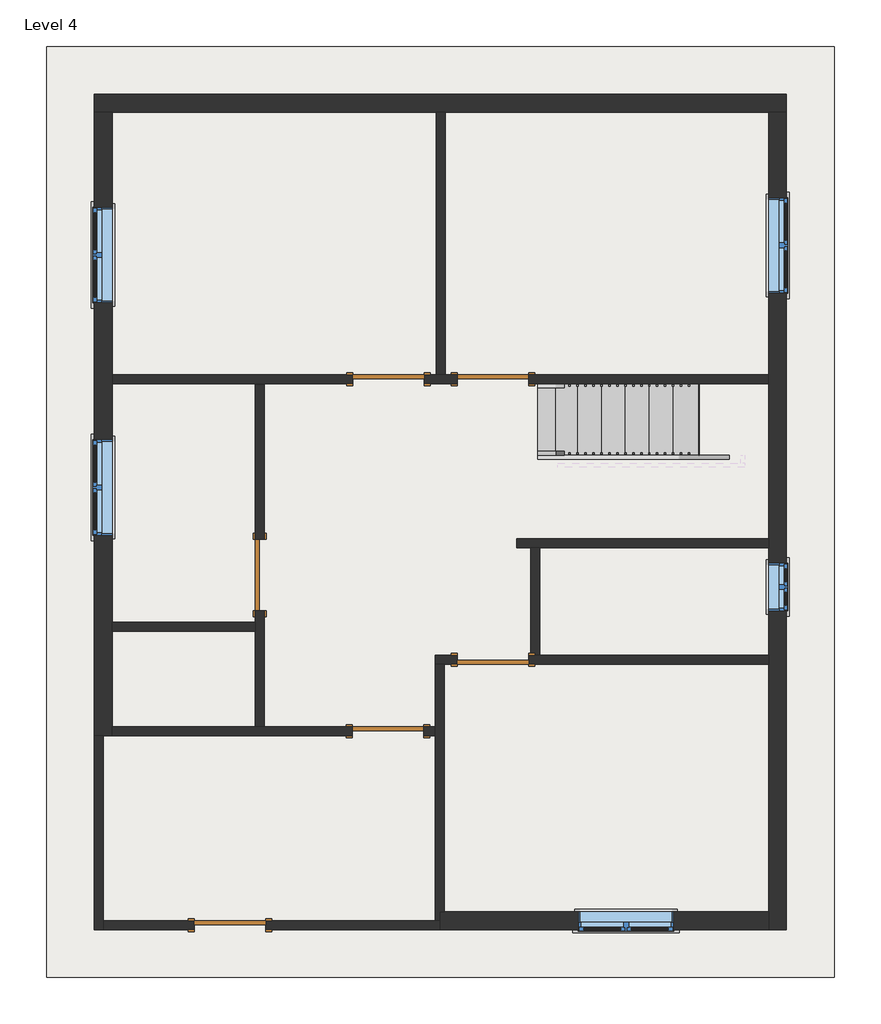
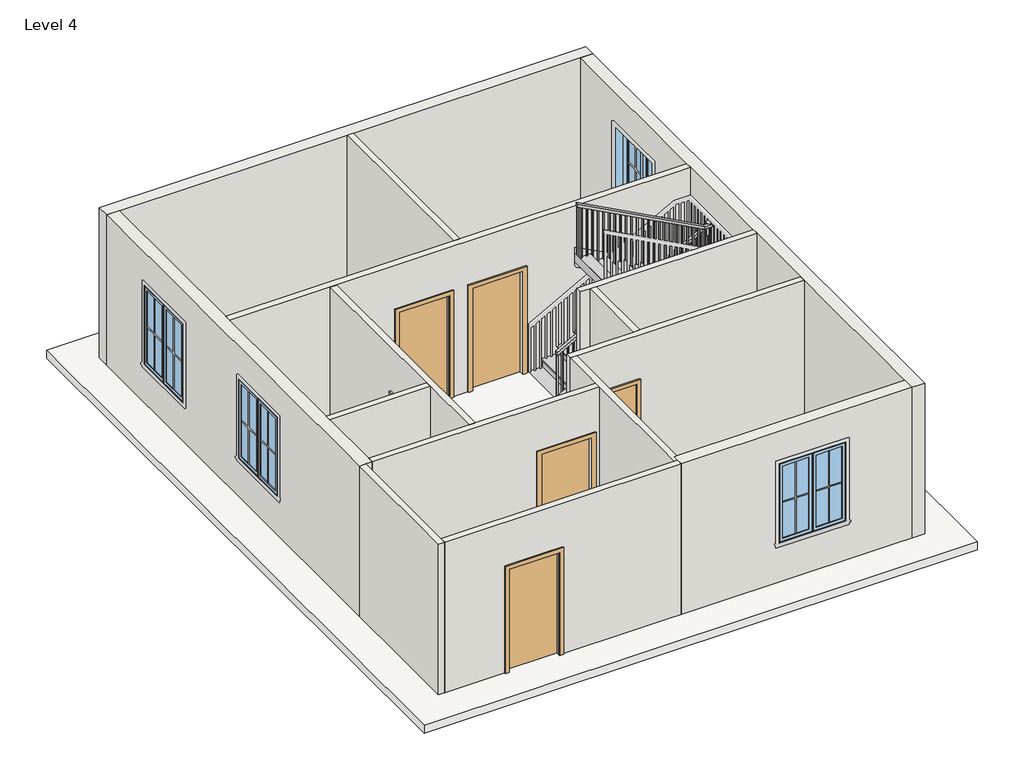
# One storey, part 1 of 2: 15 walls, 6 doors, 5 windows, 1 railing, 1 roof, 1 stair flight.
"""IFC4 building model written with IfcOpenShell, lengths in millimetres."""

from ifc_helpers import new_model, si_unit, frame, origin, place, context, project, spatial, polyline, outline, extrude, faceted_brep, transform, mapped, element, save
from components import door_305aa2a5, door_e5f9f3c4, stair_flight_cd99e03c, window_c417fced, window_8377141f

model = new_model("IFC4")

# Units and contexts
model_context = context("Model", 3, world=origin())
ifc_project = project(units=[si_unit("LENGTHUNIT", "METRE", prefix="MILLI")], contexts=[model_context])

# Site, building, storey
site = spatial("IfcSite", under=ifc_project)
building = spatial("IfcBuilding", under=site)
storey = spatial("IfcBuildingStorey", under=building, Name="Level 4", Elevation=9144.0)

# Doors
placement = place(None, origin())
door_shape = door_305aa2a5(model_context)
element("IfcDoor", 1, ObjectType="Single-Flush : 36\" x 84\"", at=placement, inside=storey, context=model_context, shape_type="MappedRepresentation", body=[
    mapped(door_shape, transform((8001.0, 9251.95, 9144.0), x_axis=(-1.0, 0.0, 0.0), y_axis=(0.0, -1.0, 0.0), z_axis=(0.0, 0.0, 1.0))),
])
element("IfcDoor", 2, ObjectType="Single-Flush : 36\" x 84\"", at=placement, inside=storey, context=model_context, shape_type="MappedRepresentation", body=[
    mapped(door_shape, transform((5022.9818578, 6750.05, 9144.0), x_axis=(0.0, -1.0, 0.0), y_axis=(1.0, 0.0, 0.0), z_axis=(0.0, 0.0, 1.0))),
])
door_2_shape = door_e5f9f3c4(model_context)
element("IfcDoor", 3, ObjectType="Single-Flush : 36\" x 84\"", at=placement, inside=storey, context=model_context, shape_type="MappedRepresentation", body=[
    mapped(door_2_shape, transform((6667.5, 9251.95, 9144.0), x_axis=(1.0, 0.0, 0.0), y_axis=(0.0, 1.0, 0.0), z_axis=(0.0, 0.0, 1.0))),
])
element("IfcDoor", 4, ObjectType="Single-Flush : 36\" x 84\"", at=placement, inside=storey, context=model_context, shape_type="MappedRepresentation", body=[
    mapped(door_2_shape, transform((8001.0, 5670.55, 9144.0), x_axis=(-1.0, 0.0, 0.0), y_axis=(0.0, -1.0, 0.0), z_axis=(0.0, 0.0, 1.0))),
])
element("IfcDoor", 5, ObjectType="Single-Flush : 36\" x 84\"", at=placement, inside=storey, context=model_context, shape_type="MappedRepresentation", body=[
    mapped(door_2_shape, transform((6658.76875, 4756.15, 9144.0), x_axis=(1.0, 0.0, 0.0), y_axis=(0.0, 1.0, 0.0), z_axis=(0.0, 0.0, 1.0))),
])
element("IfcDoor", 6, ObjectType="Single-Flush : 36\" x 84\"", at=placement, inside=storey, context=model_context, shape_type="MappedRepresentation", body=[
    mapped(door_2_shape, transform((4641.85, 2279.65, 9144.0), x_axis=(1.0, 0.0, 0.0), y_axis=(0.0, 1.0, 0.0), z_axis=(0.0, 0.0, 1.0))),
])

# Railing
element("IfcRailing", 7, ObjectType="Handrail - Rectangular", at=placement, inside=storey, context=model_context, shape_type="SolidModel", body=[
    faceted_brep([(8572.5, 8331.2, 10218.8210526), (8572.5, 8331.2, 10160.9285199), (8572.5, 8280.4, 10160.9285199), (8572.5, 8280.4, 10218.8210526), (11137.9, 8331.2, 11620.962753), (11188.7, 8331.2, 11590.8354025), (11188.7, 8280.4, 11590.8354025), (11137.9, 8280.4, 11620.962753), (11137.9, 8331.2, 11662.6105263), (11188.7, 8331.2, 11611.8105263), (11188.7, 8280.4, 11611.8105263), (11137.9, 8280.4, 11662.6105263), (11264.9, 8331.2, 11662.6105263), (11264.9, 8331.2, 11611.8105263), (11214.1, 8280.4, 11611.8105263), (11214.1, 8280.4, 11662.6105263), (11264.9, 8204.2, 11662.6105263), (11264.9, 8153.4, 11611.8105263), (11214.1, 8153.4, 11611.8105263), (11214.1, 8204.2, 11662.6105263), (11264.9, 8204.2, 11863.9901456), (11264.9, 8153.4, 11813.1901456), (11214.1, 8153.4, 11813.1901456), (11214.1, 8204.2, 11863.9901456), (11264.9, 8077.2, 11863.9901456), (11264.9, 8077.2, 11813.1901456), (11214.1, 8128.0, 11813.1901456), (11214.1, 8128.0, 11863.9901456), (11137.9, 8077.2, 11863.9901456), (11125.1122768, 8077.2, 11813.1901456), (11125.1122768, 8128.0, 11813.1901456), (11137.9, 8128.0, 11863.9901456), (8826.5, 8077.2, 13106.4), (8826.5, 8128.0, 13106.4), (8826.5, 8128.0, 13048.7264198), (8826.5, 8077.2, 13048.7264198)], [[[0, 1, 2, 3]], [[1, 0, 4, 5]], [[2, 1, 5, 6]], [[3, 2, 6, 7]], [[0, 3, 7, 4]], [[5, 4, 8, 9]], [[6, 5, 9, 10]], [[7, 6, 10, 11]], [[4, 7, 11, 8]], [[9, 8, 12, 13]], [[10, 9, 13, 14]], [[11, 10, 14, 15]], [[8, 11, 15, 12]], [[13, 12, 16, 17]], [[14, 13, 17, 18]], [[15, 14, 18, 19]], [[12, 15, 19, 16]], [[17, 16, 20, 21]], [[18, 17, 21, 22]], [[19, 18, 22, 23]], [[16, 19, 23, 20]], [[21, 20, 24, 25]], [[22, 21, 25, 26]], [[23, 22, 26, 27]], [[20, 23, 27, 24]], [[25, 24, 28, 29]], [[26, 25, 29, 30]], [[27, 26, 30, 31]], [[24, 27, 31, 28]], [[32, 33, 34, 35]], [[29, 28, 32, 35]], [[30, 29, 35, 34]], [[31, 30, 34, 33]], [[28, 31, 33, 32]]]),
    extrude(outline(polyline([(13002.6480323, 8912.225), (13012.887674, 8893.175), (12031.5789474, 8893.175), (12031.5789474, 8912.225), (13002.6480323, 8912.225)])), frame((0.0, 8093.075, 0.0), z_axis=(0.0, 1.0, 0.0), x_axis=(0.0, 0.0, 1.0)), (0.0, 0.0, 1.0), 19.05),
    extrude(outline(polyline([(12948.0366101, 9013.825), (12958.2762518, 8994.775), (12031.5789474, 8994.775), (12031.5789474, 9013.825), (12948.0366101, 9013.825)])), frame((0.0, 8093.075, 0.0), z_axis=(0.0, 1.0, 0.0), x_axis=(0.0, 0.0, 1.0)), (0.0, 0.0, 1.0), 19.05),
    extrude(outline(polyline([(12893.425188, 9115.425), (12903.6648296, 9096.375), (11871.1578947, 9096.375), (11871.1578947, 9115.425), (12893.425188, 9115.425)])), frame((0.0, 8093.075, 0.0), z_axis=(0.0, 1.0, 0.0), x_axis=(0.0, 0.0, 1.0)), (0.0, 0.0, 1.0), 19.05),
    extrude(outline(polyline([(12838.8137658, 9217.025), (12849.0534074, 9197.975), (11871.1578947, 9197.975), (11871.1578947, 9217.025), (12838.8137658, 9217.025)])), frame((0.0, 8093.075, 0.0), z_axis=(0.0, 1.0, 0.0), x_axis=(0.0, 0.0, 1.0)), (0.0, 0.0, 1.0), 19.05),
    extrude(outline(polyline([(12784.1597952, 9318.625), (12794.5717386, 9299.575), (11871.1578947, 9299.575), (11871.1578947, 9318.625), (12784.1597952, 9318.625)])), frame((0.0, 8093.075, 0.0), z_axis=(0.0, 1.0, 0.0), x_axis=(0.0, 0.0, 1.0)), (0.0, 0.0, 1.0), 19.05),
    extrude(outline(polyline([(12729.5909214, 9420.225), (12739.8305631, 9401.175), (11710.7368421, 9401.175), (11710.7368421, 9420.225), (12729.5909214, 9420.225)])), frame((0.0, 8093.075, 0.0), z_axis=(0.0, 1.0, 0.0), x_axis=(0.0, 0.0, 1.0)), (0.0, 0.0, 1.0), 19.05),
    extrude(outline(polyline([(12674.9794993, 9521.825), (12685.2191409, 9502.775), (11710.7368421, 9502.775), (11710.7368421, 9521.825), (12674.9794993, 9521.825)])), frame((0.0, 8093.075, 0.0), z_axis=(0.0, 1.0, 0.0), x_axis=(0.0, 0.0, 1.0)), (0.0, 0.0, 1.0), 19.05),
    extrude(outline(polyline([(12620.3680771, 9623.425), (12630.6077187, 9604.375), (11710.7368421, 9604.375), (11710.7368421, 9623.425), (12620.3680771, 9623.425)])), frame((0.0, 8093.075, 0.0), z_axis=(0.0, 1.0, 0.0), x_axis=(0.0, 0.0, 1.0)), (0.0, 0.0, 1.0), 19.05),
    extrude(outline(polyline([(12565.7566549, 9725.025), (12575.9962966, 9705.975), (11550.3157895, 9705.975), (11550.3157895, 9725.025), (12565.7566549, 9725.025)])), frame((0.0, 8093.075, 0.0), z_axis=(0.0, 1.0, 0.0), x_axis=(0.0, 0.0, 1.0)), (0.0, 0.0, 1.0), 19.05),
    extrude(outline(polyline([(12511.1452327, 9826.625), (12521.3848744, 9807.575), (11550.3157895, 9807.575), (11550.3157895, 9826.625), (12511.1452327, 9826.625)])), frame((0.0, 8093.075, 0.0), z_axis=(0.0, 1.0, 0.0), x_axis=(0.0, 0.0, 1.0)), (0.0, 0.0, 1.0), 19.05),
    extrude(outline(polyline([(12456.5338106, 9928.225), (12466.7734522, 9909.175), (11550.3157895, 9909.175), (11550.3157895, 9928.225), (12456.5338106, 9928.225)])), frame((0.0, 8093.075, 0.0), z_axis=(0.0, 1.0, 0.0), x_axis=(0.0, 0.0, 1.0)), (0.0, 0.0, 1.0), 19.05),
    extrude(outline(polyline([(12401.9223884, 10029.825), (12412.1620301, 10010.775), (11389.8947368, 10010.775), (11389.8947368, 10029.825), (12401.9223884, 10029.825)])), frame((0.0, 8093.075, 0.0), z_axis=(0.0, 1.0, 0.0), x_axis=(0.0, 0.0, 1.0)), (0.0, 0.0, 1.0), 19.05),
    extrude(outline(polyline([(12347.3109662, 10131.425), (12357.5506079, 10112.375), (11389.8947368, 10112.375), (11389.8947368, 10131.425), (12347.3109662, 10131.425)])), frame((0.0, 8093.075, 0.0), z_axis=(0.0, 1.0, 0.0), x_axis=(0.0, 0.0, 1.0)), (0.0, 0.0, 1.0), 19.05),
    extrude(outline(polyline([(12292.6995441, 10233.025), (12302.9391857, 10213.975), (11389.8947368, 10213.975), (11389.8947368, 10233.025), (12292.6995441, 10233.025)])), frame((0.0, 8093.075, 0.0), z_axis=(0.0, 1.0, 0.0), x_axis=(0.0, 0.0, 1.0)), (0.0, 0.0, 1.0), 19.05),
    extrude(outline(polyline([(12238.0881219, 10334.625), (12248.3277635, 10315.575), (11229.4736842, 10315.575), (11229.4736842, 10334.625), (12238.0881219, 10334.625)])), frame((0.0, 8093.075, 0.0), z_axis=(0.0, 1.0, 0.0), x_axis=(0.0, 0.0, 1.0)), (0.0, 0.0, 1.0), 19.05),
    extrude(outline(polyline([(12183.4766997, 10436.225), (12193.7163414, 10417.175), (11229.4736842, 10417.175), (11229.4736842, 10436.225), (12183.4766997, 10436.225)])), frame((0.0, 8093.075, 0.0), z_axis=(0.0, 1.0, 0.0), x_axis=(0.0, 0.0, 1.0)), (0.0, 0.0, 1.0), 19.05),
    extrude(outline(polyline([(12128.8652775, 10537.825), (12139.1049192, 10518.775), (11229.4736842, 10518.775), (11229.4736842, 10537.825), (12128.8652775, 10537.825)])), frame((0.0, 8093.075, 0.0), z_axis=(0.0, 1.0, 0.0), x_axis=(0.0, 0.0, 1.0)), (0.0, 0.0, 1.0), 19.05),
    extrude(outline(polyline([(12074.2538554, 10639.425), (12084.493497, 10620.375), (11069.0526316, 10620.375), (11069.0526316, 10639.425), (12074.2538554, 10639.425)])), frame((0.0, 8093.075, 0.0), z_axis=(0.0, 1.0, 0.0), x_axis=(0.0, 0.0, 1.0)), (0.0, 0.0, 1.0), 19.05),
    extrude(outline(polyline([(12019.6424332, 10741.025), (12029.8820749, 10721.975), (11069.0526316, 10721.975), (11069.0526316, 10741.025), (12019.6424332, 10741.025)])), frame((0.0, 8093.075, 0.0), z_axis=(0.0, 1.0, 0.0), x_axis=(0.0, 0.0, 1.0)), (0.0, 0.0, 1.0), 19.05),
    extrude(outline(polyline([(11965.031011, 10842.625), (11975.2706527, 10823.575), (11069.0526316, 10823.575), (11069.0526316, 10842.625), (11965.031011, 10842.625)])), frame((0.0, 8093.075, 0.0), z_axis=(0.0, 1.0, 0.0), x_axis=(0.0, 0.0, 1.0)), (0.0, 0.0, 1.0), 19.05),
    extrude(outline(polyline([(11910.4195889, 10944.225), (11920.6592305, 10925.175), (10908.6315789, 10925.175), (10908.6315789, 10944.225), (11910.4195889, 10944.225)])), frame((0.0, 8093.075, 0.0), z_axis=(0.0, 1.0, 0.0), x_axis=(0.0, 0.0, 1.0)), (0.0, 0.0, 1.0), 19.05),
    extrude(outline(polyline([(11855.8081667, 11045.825), (11866.0478083, 11026.775), (10908.6315789, 11026.775), (10908.6315789, 11045.825), (11855.8081667, 11045.825)])), frame((0.0, 8093.075, 0.0), z_axis=(0.0, 1.0, 0.0), x_axis=(0.0, 0.0, 1.0)), (0.0, 0.0, 1.0), 19.05),
    extrude(outline(polyline([(11801.1967445, 11147.425), (11811.4363862, 11128.375), (10908.6315789, 11128.375), (10908.6315789, 11147.425), (11801.1967445, 11147.425)])), frame((0.0, 8093.075, 0.0), z_axis=(0.0, 1.0, 0.0), x_axis=(0.0, 0.0, 1.0)), (0.0, 0.0, 1.0), 19.05),
    extrude(outline(polyline([(11229.975, 8213.725), (11249.025, 8213.725), (11249.025, 8194.675), (11229.975, 8194.675), (11229.975, 8213.725)])), frame((0.0, 0.0, 10748.2105263), z_axis=(0.0, 0.0, 1.0), x_axis=(1.0, 0.0, 0.0)), (0.0, 0.0, 1.0), 863.6),
    extrude(outline(polyline([(11204.575, 8296.275), (11204.575, 8315.325), (11223.625, 8315.325), (11223.625, 8296.275), (11204.575, 8296.275)])), frame((0.0, 0.0, 10748.2105263), z_axis=(0.0, 0.0, 1.0), x_axis=(1.0, 0.0, 0.0)), (0.0, 0.0, 1.0), 863.6),
    extrude(outline(polyline([(11554.3936009, 11122.025), (11543.9816576, 11102.975), (10587.7894737, 11102.975), (10587.7894737, 11122.025), (11554.3936009, 11122.025)])), frame((0.0, 8296.275, 0.0), z_axis=(0.0, 1.0, 0.0), x_axis=(0.0, 0.0, 1.0)), (0.0, 0.0, 1.0), 19.05),
    extrude(outline(polyline([(11498.8632365, 11020.425), (11488.4512932, 11001.375), (10587.7894737, 11001.375), (10587.7894737, 11020.425), (11498.8632365, 11020.425)])), frame((0.0, 8296.275, 0.0), z_axis=(0.0, 1.0, 0.0), x_axis=(0.0, 0.0, 1.0)), (0.0, 0.0, 1.0), 19.05),
    extrude(outline(polyline([(11443.3328722, 10918.825), (11432.9209288, 10899.775), (10587.7894737, 10899.775), (10587.7894737, 10918.825), (11443.3328722, 10918.825)])), frame((0.0, 8296.275, 0.0), z_axis=(0.0, 1.0, 0.0), x_axis=(0.0, 0.0, 1.0)), (0.0, 0.0, 1.0), 19.05),
    extrude(outline(polyline([(11387.8025078, 10817.225), (11377.3905645, 10798.175), (10427.3684211, 10798.175), (10427.3684211, 10817.225), (11387.8025078, 10817.225)])), frame((0.0, 8296.275, 0.0), z_axis=(0.0, 1.0, 0.0), x_axis=(0.0, 0.0, 1.0)), (0.0, 0.0, 1.0), 19.05),
    extrude(outline(polyline([(11332.2721434, 10715.625), (11321.8602001, 10696.575), (10427.3684211, 10696.575), (10427.3684211, 10715.625), (11332.2721434, 10715.625)])), frame((0.0, 8296.275, 0.0), z_axis=(0.0, 1.0, 0.0), x_axis=(0.0, 0.0, 1.0)), (0.0, 0.0, 1.0), 19.05),
    extrude(outline(polyline([(11276.741779, 10614.025), (11266.3298357, 10594.975), (10427.3684211, 10594.975), (10427.3684211, 10614.025), (11276.741779, 10614.025)])), frame((0.0, 8296.275, 0.0), z_axis=(0.0, 1.0, 0.0), x_axis=(0.0, 0.0, 1.0)), (0.0, 0.0, 1.0), 19.05),
    extrude(outline(polyline([(11221.2114147, 10512.425), (11210.7994714, 10493.375), (10266.9473684, 10493.375), (10266.9473684, 10512.425), (11221.2114147, 10512.425)])), frame((0.0, 8296.275, 0.0), z_axis=(0.0, 1.0, 0.0), x_axis=(0.0, 0.0, 1.0)), (0.0, 0.0, 1.0), 19.05),
    extrude(outline(polyline([(11165.6810503, 10410.825), (11155.269107, 10391.775), (10266.9473684, 10391.775), (10266.9473684, 10410.825), (11165.6810503, 10410.825)])), frame((0.0, 8296.275, 0.0), z_axis=(0.0, 1.0, 0.0), x_axis=(0.0, 0.0, 1.0)), (0.0, 0.0, 1.0), 19.05),
    extrude(outline(polyline([(11110.1506859, 10309.225), (11099.7387426, 10290.175), (10266.9473684, 10290.175), (10266.9473684, 10309.225), (11110.1506859, 10309.225)])), frame((0.0, 8296.275, 0.0), z_axis=(0.0, 1.0, 0.0), x_axis=(0.0, 0.0, 1.0)), (0.0, 0.0, 1.0), 19.05),
    extrude(outline(polyline([(11054.6203216, 10207.625), (11044.2083782, 10188.575), (10106.5263158, 10188.575), (10106.5263158, 10207.625), (11054.6203216, 10207.625)])), frame((0.0, 8296.275, 0.0), z_axis=(0.0, 1.0, 0.0), x_axis=(0.0, 0.0, 1.0)), (0.0, 0.0, 1.0), 19.05),
    extrude(outline(polyline([(10999.0899572, 10106.025), (10988.6780139, 10086.975), (10106.5263158, 10086.975), (10106.5263158, 10106.025), (10999.0899572, 10106.025)])), frame((0.0, 8296.275, 0.0), z_axis=(0.0, 1.0, 0.0), x_axis=(0.0, 0.0, 1.0)), (0.0, 0.0, 1.0), 19.05),
    extrude(outline(polyline([(10943.5595928, 10004.425), (10933.1476495, 9985.375), (10106.5263158, 9985.375), (10106.5263158, 10004.425), (10943.5595928, 10004.425)])), frame((0.0, 8296.275, 0.0), z_axis=(0.0, 1.0, 0.0), x_axis=(0.0, 0.0, 1.0)), (0.0, 0.0, 1.0), 19.05),
    extrude(outline(polyline([(10888.0292284, 9902.825), (10877.6172851, 9883.775), (9946.1052632, 9883.775), (9946.1052632, 9902.825), (10888.0292284, 9902.825)])), frame((0.0, 8296.275, 0.0), z_axis=(0.0, 1.0, 0.0), x_axis=(0.0, 0.0, 1.0)), (0.0, 0.0, 1.0), 19.05),
    extrude(outline(polyline([(10832.4988641, 9801.225), (10822.0869207, 9782.175), (9946.1052632, 9782.175), (9946.1052632, 9801.225), (10832.4988641, 9801.225)])), frame((0.0, 8296.275, 0.0), z_axis=(0.0, 1.0, 0.0), x_axis=(0.0, 0.0, 1.0)), (0.0, 0.0, 1.0), 19.05),
    extrude(outline(polyline([(10776.9684997, 9699.625), (10766.5565564, 9680.575), (9946.1052632, 9680.575), (9946.1052632, 9699.625), (10776.9684997, 9699.625)])), frame((0.0, 8296.275, 0.0), z_axis=(0.0, 1.0, 0.0), x_axis=(0.0, 0.0, 1.0)), (0.0, 0.0, 1.0), 19.05),
    extrude(outline(polyline([(10721.4381353, 9598.025), (10711.026192, 9578.975), (9785.6842105, 9578.975), (9785.6842105, 9598.025), (10721.4381353, 9598.025)])), frame((0.0, 8296.275, 0.0), z_axis=(0.0, 1.0, 0.0), x_axis=(0.0, 0.0, 1.0)), (0.0, 0.0, 1.0), 19.05),
    extrude(outline(polyline([(10665.9077709, 9496.425), (10655.4958276, 9477.375), (9785.6842105, 9477.375), (9785.6842105, 9496.425), (10665.9077709, 9496.425)])), frame((0.0, 8296.275, 0.0), z_axis=(0.0, 1.0, 0.0), x_axis=(0.0, 0.0, 1.0)), (0.0, 0.0, 1.0), 19.05),
    extrude(outline(polyline([(10610.3774066, 9394.825), (10599.9654633, 9375.775), (9785.6842105, 9375.775), (9785.6842105, 9394.825), (10610.3774066, 9394.825)])), frame((0.0, 8296.275, 0.0), z_axis=(0.0, 1.0, 0.0), x_axis=(0.0, 0.0, 1.0)), (0.0, 0.0, 1.0), 19.05),
    extrude(outline(polyline([(10554.8470422, 9293.225), (10544.4350989, 9274.175), (9625.2631579, 9274.175), (9625.2631579, 9293.225), (10554.8470422, 9293.225)])), frame((0.0, 8296.275, 0.0), z_axis=(0.0, 1.0, 0.0), x_axis=(0.0, 0.0, 1.0)), (0.0, 0.0, 1.0), 19.05),
    extrude(outline(polyline([(10499.3166778, 9191.625), (10488.9047345, 9172.575), (9625.2631579, 9172.575), (9625.2631579, 9191.625), (10499.3166778, 9191.625)])), frame((0.0, 8296.275, 0.0), z_axis=(0.0, 1.0, 0.0), x_axis=(0.0, 0.0, 1.0)), (0.0, 0.0, 1.0), 19.05),
    extrude(outline(polyline([(10443.7863135, 9090.025), (10433.3743701, 9070.975), (9625.2631579, 9070.975), (9625.2631579, 9090.025), (10443.7863135, 9090.025)])), frame((0.0, 8296.275, 0.0), z_axis=(0.0, 1.0, 0.0), x_axis=(0.0, 0.0, 1.0)), (0.0, 0.0, 1.0), 19.05),
    extrude(outline(polyline([(10388.2559491, 8988.425), (10377.8440058, 8969.375), (9464.8421053, 8969.375), (9464.8421053, 8988.425), (10388.2559491, 8988.425)])), frame((0.0, 8296.275, 0.0), z_axis=(0.0, 1.0, 0.0), x_axis=(0.0, 0.0, 1.0)), (0.0, 0.0, 1.0), 19.05),
    extrude(outline(polyline([(10332.7255847, 8886.825), (10322.3136414, 8867.775), (9464.8421053, 8867.775), (9464.8421053, 8886.825), (10332.7255847, 8886.825)])), frame((0.0, 8296.275, 0.0), z_axis=(0.0, 1.0, 0.0), x_axis=(0.0, 0.0, 1.0)), (0.0, 0.0, 1.0), 19.05),
    extrude(outline(polyline([(10277.1952203, 8785.225), (10266.783277, 8766.175), (9304.4210526, 8766.175), (9304.4210526, 8785.225), (10277.1952203, 8785.225)])), frame((0.0, 8296.275, 0.0), z_axis=(0.0, 1.0, 0.0), x_axis=(0.0, 0.0, 1.0)), (0.0, 0.0, 1.0), 19.05),
    extrude(outline(polyline([(10221.664856, 8683.625), (10211.2529126, 8664.575), (9304.4210526, 8664.575), (9304.4210526, 8683.625), (10221.664856, 8683.625)])), frame((0.0, 8296.275, 0.0), z_axis=(0.0, 1.0, 0.0), x_axis=(0.0, 0.0, 1.0)), (0.0, 0.0, 1.0), 19.05),
    extrude(outline(polyline([(11229.975, 8112.125), (11249.025, 8112.125), (11249.025, 8093.075), (11229.975, 8093.075), (11229.975, 8112.125)])), frame((0.0, 0.0, 10748.2105263), z_axis=(0.0, 0.0, 1.0), x_axis=(1.0, 0.0, 0.0)), (0.0, 0.0, 1.0), 1064.9796193),
    extrude(outline(polyline([(11229.975, 8296.275), (11229.975, 8315.325), (11249.025, 8315.325), (11249.025, 8296.275), (11229.975, 8296.275)])), frame((0.0, 0.0, 10748.2105263), z_axis=(0.0, 0.0, 1.0), x_axis=(1.0, 0.0, 0.0)), (0.0, 0.0, 1.0), 863.6),
    extrude(outline(polyline([(13038.4867781, 8845.55), (13048.7264198, 8826.5), (12031.5789474, 8826.5), (12031.5789474, 8845.55), (13038.4867781, 8845.55)])), frame((0.0, 8093.075, 0.0), z_axis=(0.0, 1.0, 0.0), x_axis=(0.0, 0.0, 1.0)), (0.0, 0.0, 1.0), 19.05),
    extrude(outline(polyline([(10171.3404633, 8591.55), (10160.9285199, 8572.5), (9304.4210526, 8572.5), (9304.4210526, 8591.55), (10171.3404633, 8591.55)])), frame((0.0, 8296.275, 0.0), z_axis=(0.0, 1.0, 0.0), x_axis=(0.0, 0.0, 1.0)), (0.0, 0.0, 1.0), 19.05),
])

# Roof
element("IfcRoof", 8, ObjectType="Generic - 12\"", at=placement, inside=storey, context=model_context, shape_type="SweptSolid", body=[
    extrude(outline(polyline([(2298.7, 13500.1), (12357.1, 13500.1), (12357.1, 1612.9), (2298.7, 1612.9), (2298.7, 13500.1)])), frame((0.0, 0.0, 9144.0), z_axis=(0.0, 0.0, 1.0), x_axis=(1.0, 0.0, 0.0)), (0.0, 0.0, 1.0), 152.4),
])

# Stair flight
stair_flight_shape = stair_flight_cd99e03c(model_context)
element("IfcStairFlight", 9, ObjectType="2\" Tread 1\" Nosing 1/4\" Riser", at=placement, inside=storey, context=model_context, shape_type="MappedRepresentation", body=[
    mapped(stair_flight_shape, transform((0.0, 0.0, 0.0), x_axis=(1.0, 0.0, 0.0), y_axis=(0.0, 1.0, 0.0), z_axis=(0.0, 0.0, 1.0))),
])

# Walls
element("IfcWall", 10, ObjectType="Generic - 5\"", at=placement, inside=storey, context=model_context, shape_type="Brep", body=[
    faceted_brep([(7115.96875, 4699.0, 11277.6), (7115.96875, 4699.0, 9144.0), (7264.4, 4699.0, 9144.0), (7264.4, 4699.0, 12192.0), (3136.9, 4699.0, 12192.0), (3136.9, 4699.0, 9144.0), (6201.56875, 4699.0, 9144.0), (6201.56875, 4699.0, 11277.6), (7264.4, 4813.3, 9144.0), (7115.96875, 4813.3, 9144.0), (7115.96875, 4813.3, 11277.6), (6201.56875, 4813.3, 11277.6), (6201.56875, 4813.3, 9144.0), (5080.1318578, 4813.3, 9144.0), (4965.8318578, 4813.3, 9144.0), (3136.9, 4813.3, 9144.0), (3136.9, 4813.3, 12192.0), (4965.8318578, 4813.3, 12192.0), (5080.1318578, 4813.3, 12192.0), (7264.4, 4813.3, 12192.0)], [[[0, 1, 2, 3, 4, 5, 6, 7]], [[8, 9, 10, 11, 12, 13, 14, 15, 16, 17, 18, 19]], [[6, 5, 15, 14, 13, 12]], [[2, 1, 9, 8]], [[4, 3, 19, 18, 17, 16]], [[5, 4, 16, 15]], [[3, 2, 8, 19]], [[10, 9, 1, 0]], [[11, 10, 0, 7]], [[12, 11, 7, 6]]]),
])
element("IfcWall", 11, ObjectType="Generic - 5\"", at=placement, inside=storey, context=model_context, shape_type="SweptSolid", body=[
    extrude(outline(polyline([(4965.8318578, 6032.5), (3136.9, 6032.5), (3136.9, 6146.8), (4965.8318578, 6146.8), (4965.8318578, 6032.5)])), frame((0.0, 0.0, 9144.0), z_axis=(0.0, 0.0, 1.0), x_axis=(1.0, 0.0, 0.0)), (0.0, 0.0, 1.0), 3048.0),
])
element("IfcWall", 12, ObjectType="Generic - 5\"", at=placement, inside=storey, context=model_context, shape_type="Brep", body=[
    faceted_brep([(5080.1318578, 4813.3, 9144.0), (5080.1318578, 6292.85, 9144.0), (5080.1318578, 6292.85, 11277.6), (5080.1318578, 7207.25, 11277.6), (5080.1318578, 7207.25, 9144.0), (5080.1318578, 9182.1, 9144.0), (5080.1318578, 9182.1, 12192.0), (5080.1318578, 4813.3, 12192.0), (4965.8318578, 6292.85, 11277.6), (4965.8318578, 6292.85, 9144.0), (4965.8318578, 6146.8, 9144.0), (4965.8318578, 6032.5, 9144.0), (4965.8318578, 4813.3, 9144.0), (4965.8318578, 4813.3, 12192.0), (4965.8318578, 6032.5, 12192.0), (4965.8318578, 6146.8, 12192.0), (4965.8318578, 9182.1, 12192.0), (4965.8318578, 9182.1, 9144.0), (4965.8318578, 7207.25, 9144.0), (4965.8318578, 7207.25, 11277.6)], [[[0, 1, 2, 3, 4, 5, 6, 7]], [[8, 9, 10, 11, 12, 13, 14, 15, 16, 17, 18, 19]], [[18, 17, 5, 4]], [[12, 11, 10, 9, 1, 0]], [[6, 5, 17, 16]], [[7, 6, 16, 15, 14, 13]], [[0, 7, 13, 12]], [[2, 1, 9, 8]], [[3, 2, 8, 19]], [[4, 3, 19, 18]]]),
])
element("IfcWall", 13, ObjectType="Generic - 5\"", at=placement, inside=storey, context=model_context, shape_type="Brep", body=[
    faceted_brep([(7124.7, 9194.8, 11277.6), (7124.7, 9194.8, 9144.0), (7543.8, 9194.8, 9144.0), (7543.8, 9194.8, 11277.6), (8458.2, 9194.8, 11277.6), (8458.2, 9194.8, 9144.0), (11518.9, 9194.8, 9144.0), (11518.9, 9194.8, 12192.0), (3136.9, 9194.8, 12192.0), (3136.9, 9194.8, 9144.0), (6210.3, 9194.8, 9144.0), (6210.3, 9194.8, 11277.6), (7543.8, 9309.1, 9144.0), (7391.4, 9309.1, 9144.0), (7277.1, 9309.1, 9144.0), (7124.7, 9309.1, 9144.0), (7124.7, 9309.1, 11277.6), (6210.3, 9309.1, 11277.6), (6210.3, 9309.1, 9144.0), (3136.9, 9309.1, 9144.0), (3136.9, 9309.1, 12192.0), (7277.1, 9309.1, 12192.0), (7391.4, 9309.1, 12192.0), (11518.9, 9309.1, 12192.0), (11518.9, 9309.1, 9144.0), (8458.2, 9309.1, 9144.0), (8458.2, 9309.1, 11277.6), (7543.8, 9309.1, 11277.6)], [[[0, 1, 2, 3, 4, 5, 6, 7, 8, 9, 10, 11]], [[12, 13, 14, 15, 16, 17, 18, 19, 20, 21, 22, 23, 24, 25, 26, 27]], [[25, 24, 6, 5]], [[10, 9, 19, 18]], [[2, 1, 15, 14, 13, 12]], [[8, 7, 23, 22, 21, 20]], [[7, 6, 24, 23]], [[9, 8, 20, 19]], [[3, 2, 12, 27]], [[4, 3, 27, 26]], [[5, 4, 26, 25]], [[16, 15, 1, 0]], [[17, 16, 0, 11]], [[18, 17, 11, 10]]]),
])
element("IfcWall", 14, ObjectType="Generic - 5\"", at=placement, inside=storey, context=model_context, shape_type="SweptSolid", body=[
    extrude(outline(polyline([(7277.1, 9309.1), (7277.1, 12661.9), (7391.4, 12661.9), (7391.4, 9309.1), (7277.1, 9309.1)])), frame((0.0, 0.0, 9144.0), z_axis=(0.0, 0.0, 1.0), x_axis=(1.0, 0.0, 0.0)), (0.0, 0.0, 1.0), 3048.0),
])
element("IfcWall", 15, ObjectType="Generic - 5\"", at=placement, inside=storey, context=model_context, shape_type="Brep", body=[
    faceted_brep([(2908.3, 4699.0, 9144.0), (2908.3, 2222.5, 9144.0), (2908.3, 2222.5, 12192.0), (2908.3, 4699.0, 12192.0), (3022.6, 4699.0, 9144.0), (3022.6, 4699.0, 12192.0), (3022.6, 2336.8, 12192.0), (3022.6, 2222.5, 12192.0), (3022.6, 2222.5, 9144.0), (3022.6, 2336.8, 9144.0)], [[[0, 1, 2, 3]], [[4, 5, 6, 7, 8, 9]], [[1, 0, 4, 9, 8]], [[3, 2, 7, 6, 5]], [[0, 3, 5, 4]], [[2, 1, 8, 7]]]),
])
element("IfcWall", 16, ObjectType="Generic - 5\"", at=placement, inside=storey, context=model_context, shape_type="Brep", body=[
    faceted_brep([(5099.05, 2222.5, 11277.6), (5099.05, 2222.5, 9144.0), (7321.55, 2222.5, 9144.0), (7321.55, 2222.5, 12192.0), (3022.6, 2222.5, 12192.0), (3022.6, 2222.5, 9144.0), (4184.65, 2222.5, 9144.0), (4184.65, 2222.5, 11277.6), (7321.55, 2336.8, 9144.0), (7264.4, 2336.8, 9144.0), (5099.05, 2336.8, 9144.0), (5099.05, 2336.8, 11277.6), (4184.65, 2336.8, 11277.6), (4184.65, 2336.8, 9144.0), (3022.6, 2336.8, 9144.0), (3022.6, 2336.8, 12192.0), (7264.4, 2336.8, 12192.0), (7321.55, 2336.8, 12192.0)], [[[0, 1, 2, 3, 4, 5, 6, 7]], [[8, 9, 10, 11, 12, 13, 14, 15, 16, 17]], [[6, 5, 14, 13]], [[2, 1, 10, 9, 8]], [[3, 2, 8, 17]], [[4, 3, 17, 16, 15]], [[5, 4, 15, 14]], [[11, 10, 1, 0]], [[12, 11, 0, 7]], [[13, 12, 7, 6]]]),
])
element("IfcWall", 17, ObjectType="Generic - 5\"", at=placement, inside=storey, context=model_context, shape_type="Brep", body=[
    faceted_brep([(11518.9, 7213.6, 9144.0), (8305.8, 7213.6, 9144.0), (8305.8, 7213.6, 12192.0), (11518.9, 7213.6, 12192.0), (11518.9, 7099.3, 9144.0), (11518.9, 7099.3, 12192.0), (8597.9, 7099.3, 12192.0), (8483.6, 7099.3, 12192.0), (8305.8, 7099.3, 12192.0), (8305.8, 7099.3, 9144.0), (8483.6, 7099.3, 9144.0), (8597.9, 7099.3, 9144.0)], [[[0, 1, 2, 3]], [[4, 5, 6, 7, 8, 9, 10, 11]], [[1, 0, 4, 11, 10, 9]], [[2, 1, 9, 8]], [[3, 2, 8, 7, 6, 5]], [[0, 3, 5, 4]]]),
])
element("IfcWall", 18, ObjectType="Generic - 5\"", at=placement, inside=storey, context=model_context, shape_type="SweptSolid", body=[
    extrude(outline(polyline([(8483.6, 5727.7), (8483.6, 7099.3), (8597.9, 7099.3), (8597.9, 5727.7), (8483.6, 5727.7)])), frame((0.0, 0.0, 9144.0), z_axis=(0.0, 0.0, 1.0), x_axis=(1.0, 0.0, 0.0)), (0.0, 0.0, 1.0), 3048.0),
])
element("IfcWall", 19, ObjectType="Generic - 5\"", at=placement, inside=storey, context=model_context, shape_type="Brep", body=[
    faceted_brep([(7543.8, 5727.7, 11277.6), (7543.8, 5727.7, 9144.0), (7264.4, 5727.7, 9144.0), (7264.4, 5727.7, 12192.0), (8483.6, 5727.7, 12192.0), (8597.9, 5727.7, 12192.0), (11518.9, 5727.7, 12192.0), (11518.9, 5727.7, 9144.0), (8597.9, 5727.7, 9144.0), (8483.6, 5727.7, 9144.0), (8458.2, 5727.7, 9144.0), (8458.2, 5727.7, 11277.6), (7264.4, 5613.4, 9144.0), (7378.7, 5613.4, 9144.0), (7543.8, 5613.4, 9144.0), (7543.8, 5613.4, 11277.6), (8458.2, 5613.4, 11277.6), (8458.2, 5613.4, 9144.0), (11518.9, 5613.4, 9144.0), (11518.9, 5613.4, 12192.0), (7378.7, 5613.4, 12192.0), (7264.4, 5613.4, 12192.0)], [[[0, 1, 2, 3, 4, 5, 6, 7, 8, 9, 10, 11]], [[12, 13, 14, 15, 16, 17, 18, 19, 20, 21]], [[2, 1, 14, 13, 12]], [[10, 9, 8, 7, 18, 17]], [[6, 5, 4, 3, 21, 20, 19]], [[7, 6, 19, 18]], [[3, 2, 12, 21]], [[15, 14, 1, 0]], [[16, 15, 0, 11]], [[17, 16, 11, 10]]]),
])
element("IfcWall", 20, ObjectType="Generic - 5\"", at=placement, inside=storey, context=model_context, shape_type="Brep", body=[
    faceted_brep([(7264.4, 5613.4, 9144.0), (7264.4, 4813.3, 9144.0), (7264.4, 4699.0, 9144.0), (7264.4, 2336.8, 9144.0), (7264.4, 2336.8, 12192.0), (7264.4, 4699.0, 12192.0), (7264.4, 4813.3, 12192.0), (7264.4, 5613.4, 12192.0), (7378.7, 5613.4, 9144.0), (7378.7, 5613.4, 12192.0), (7378.7, 2451.1, 12192.0), (7378.7, 2451.1, 9144.0), (7321.55, 2451.1, 9144.0), (7321.55, 2336.8, 9144.0), (7321.55, 2336.8, 12192.0), (7321.55, 2451.1, 12192.0)], [[[0, 1, 2, 3, 4, 5, 6, 7]], [[8, 9, 10, 11]], [[3, 2, 1, 0, 8, 11, 12, 13]], [[7, 6, 5, 4, 14, 15, 10, 9]], [[0, 7, 9, 8]], [[4, 3, 13, 14]], [[13, 12, 15, 14]], [[12, 11, 10, 15]]]),
])
element("IfcWall", 21, ObjectType="Generic - 8\"", at=placement, inside=storey, context=model_context, shape_type="Brep", body=[
    faceted_brep([(2908.3, 12661.9, 9144.0), (3136.9, 12661.9, 9144.0), (7277.1, 12661.9, 9144.0), (7391.4, 12661.9, 9144.0), (11518.9, 12661.9, 9144.0), (11747.5, 12661.9, 9144.0), (11747.5, 12661.9, 12192.0), (11518.9, 12661.9, 12192.0), (7391.4, 12661.9, 12192.0), (7277.1, 12661.9, 12192.0), (3136.9, 12661.9, 12192.0), (2908.3, 12661.9, 12192.0), (2908.3, 12890.5, 9144.0), (2908.3, 12890.5, 12192.0), (11747.5, 12890.5, 12192.0), (11747.5, 12890.5, 9144.0)], [[[0, 1, 2, 3, 4, 5, 6, 7, 8, 9, 10, 11]], [[12, 13, 14, 15]], [[5, 4, 3, 2, 1, 0, 12, 15]], [[11, 10, 9, 8, 7, 6, 14, 13]], [[6, 5, 15, 14]], [[0, 11, 13, 12]]]),
])
element("IfcWall", 22, ObjectType="Generic - 8\"", at=placement, inside=storey, context=model_context, shape_type="Brep", body=[
    faceted_brep([(11518.9, 12661.9, 9144.0), (11518.9, 9309.1, 9144.0), (11518.9, 9194.8, 9144.0), (11518.9, 7213.6, 9144.0), (11518.9, 7099.3, 9144.0), (11518.9, 5727.7, 9144.0), (11518.9, 5613.4, 9144.0), (11518.9, 2451.1, 9144.0), (11518.9, 2222.5, 9144.0), (11518.9, 2222.5, 12192.0), (11518.9, 2451.1, 12192.0), (11518.9, 5613.4, 12192.0), (11518.9, 5727.7, 12192.0), (11518.9, 7099.3, 12192.0), (11518.9, 7213.6, 12192.0), (11518.9, 9194.8, 12192.0), (11518.9, 9309.1, 12192.0), (11518.9, 12661.9, 12192.0), (11518.9, 10352.0875, 11582.4), (11518.9, 10352.0875, 10058.4), (11518.9, 11571.2875, 10058.4), (11518.9, 11571.2875, 11582.4), (11518.9, 6292.85, 10972.8), (11518.9, 6292.85, 10058.4), (11518.9, 6902.45, 10058.4), (11518.9, 6902.45, 10972.8), (11747.5, 12661.9, 9144.0), (11747.5, 12661.9, 12192.0), (11747.5, 2222.5, 12192.0), (11747.5, 2222.5, 9144.0), (11747.5, 10352.0875, 11582.4), (11747.5, 11571.2875, 11582.4), (11747.5, 11571.2875, 10058.4), (11747.5, 10352.0875, 10058.4), (11747.5, 6292.85, 10972.8), (11747.5, 6902.45, 10972.8), (11747.5, 6902.45, 10058.4), (11747.5, 6292.85, 10058.4)], [[[0, 1, 2, 3, 4, 5, 6, 7, 8, 9, 10, 11, 12, 13, 14, 15, 16, 17], [18, 19, 20, 21], [22, 23, 24, 25]], [[26, 27, 28, 29], [30, 31, 32, 33], [34, 35, 36, 37]], [[8, 7, 6, 5, 4, 3, 2, 1, 0, 26, 29]], [[17, 16, 15, 14, 13, 12, 11, 10, 9, 28, 27]], [[0, 17, 27, 26]], [[9, 8, 29, 28]], [[19, 18, 30, 33]], [[20, 19, 33, 32]], [[21, 20, 32, 31]], [[18, 21, 31, 30]], [[23, 22, 34, 37]], [[24, 23, 37, 36]], [[25, 24, 36, 35]], [[22, 25, 35, 34]]]),
])
element("IfcWall", 23, ObjectType="Generic - 8\"", at=placement, inside=storey, context=model_context, shape_type="Brep", body=[
    faceted_brep([(2908.3, 12661.9, 9144.0), (2908.3, 4699.0, 9144.0), (2908.3, 4699.0, 12192.0), (2908.3, 12661.9, 12192.0), (2908.3, 8480.425, 11582.4), (2908.3, 7261.225, 11582.4), (2908.3, 7261.225, 10058.4), (2908.3, 8480.425, 10058.4), (2908.3, 11449.05, 11582.4), (2908.3, 10229.85, 11582.4), (2908.3, 10229.85, 10058.4), (2908.3, 11449.05, 10058.4), (3136.9, 12661.9, 9144.0), (3136.9, 12661.9, 12192.0), (3136.9, 9309.1, 12192.0), (3136.9, 9194.8, 12192.0), (3136.9, 6146.8, 12192.0), (3136.9, 6032.5, 12192.0), (3136.9, 4813.3, 12192.0), (3136.9, 4699.0, 12192.0), (3136.9, 4699.0, 9144.0), (3136.9, 4813.3, 9144.0), (3136.9, 6032.5, 9144.0), (3136.9, 6146.8, 9144.0), (3136.9, 9194.8, 9144.0), (3136.9, 9309.1, 9144.0), (3136.9, 8480.425, 11582.4), (3136.9, 8480.425, 10058.4), (3136.9, 7261.225, 10058.4), (3136.9, 7261.225, 11582.4), (3136.9, 11449.05, 11582.4), (3136.9, 11449.05, 10058.4), (3136.9, 10229.85, 10058.4), (3136.9, 10229.85, 11582.4), (3022.6, 4699.0, 9144.0), (3022.6, 4699.0, 12192.0)], [[[0, 1, 2, 3], [4, 5, 6, 7], [8, 9, 10, 11]], [[12, 13, 14, 15, 16, 17, 18, 19, 20, 21, 22, 23, 24, 25], [26, 27, 28, 29], [30, 31, 32, 33]], [[1, 0, 12, 25, 24, 23, 22, 21, 20, 34]], [[3, 2, 35, 19, 18, 17, 16, 15, 14, 13]], [[0, 3, 13, 12]], [[2, 1, 34, 20, 19, 35]], [[27, 26, 4, 7]], [[28, 27, 7, 6]], [[29, 28, 6, 5]], [[26, 29, 5, 4]], [[31, 30, 8, 11]], [[32, 31, 11, 10]], [[33, 32, 10, 9]], [[30, 33, 9, 8]]]),
])
element("IfcWall", 24, ObjectType="Generic - 8\"", at=placement, inside=storey, context=model_context, shape_type="Brep", body=[
    faceted_brep([(7321.55, 2222.5, 9144.0), (11518.9, 2222.5, 9144.0), (11518.9, 2222.5, 12192.0), (7321.55, 2222.5, 12192.0), (9090.81875, 2222.5, 11582.4), (10310.01875, 2222.5, 11582.4), (10310.01875, 2222.5, 10058.4), (9090.81875, 2222.5, 10058.4), (7321.55, 2451.1, 9144.0), (7321.55, 2451.1, 12192.0), (7378.7, 2451.1, 12192.0), (11518.9, 2451.1, 12192.0), (11518.9, 2451.1, 9144.0), (7378.7, 2451.1, 9144.0), (9090.81875, 2451.1, 11582.4), (9090.81875, 2451.1, 10058.4), (10310.01875, 2451.1, 10058.4), (10310.01875, 2451.1, 11582.4), (7321.55, 2336.8, 9144.0), (7321.55, 2336.8, 12192.0)], [[[0, 1, 2, 3], [4, 5, 6, 7]], [[8, 9, 10, 11, 12, 13], [14, 15, 16, 17]], [[1, 0, 18, 8, 13, 12]], [[3, 2, 11, 10, 9, 19]], [[0, 3, 19, 9, 8, 18]], [[2, 1, 12, 11]], [[15, 14, 4, 7]], [[16, 15, 7, 6]], [[17, 16, 6, 5]], [[14, 17, 5, 4]]]),
])

# Windows
window_shape = window_c417fced(model_context)
element("IfcWindow", 25, ObjectType="Window-Casement-Double : 24\" x 36\"", at=placement, inside=storey, context=model_context, shape_type="MappedRepresentation", body=[
    mapped(window_shape, transform((11633.2, 6597.65, 9144.0), x_axis=(0.0, -1.0, 0.0), y_axis=(1.0, 0.0, 0.0), z_axis=(0.0, 0.0, 1.0))),
])
window_2_shape = window_8377141f(model_context)
element("IfcWindow", 26, ObjectType="Window-Casement-Double : 48\" x 60\"", at=placement, inside=storey, context=model_context, shape_type="MappedRepresentation", body=[
    mapped(window_2_shape, transform((9700.41875, 2336.8, 9144.0), x_axis=(-1.0, 0.0, 0.0), y_axis=(0.0, -1.0, 0.0), z_axis=(0.0, 0.0, 1.0))),
])
element("IfcWindow", 27, ObjectType="Window-Casement-Double : 48\" x 60\"", at=placement, inside=storey, context=model_context, shape_type="MappedRepresentation", body=[
    mapped(window_2_shape, transform((3022.6, 7870.825, 9144.0), x_axis=(0.0, 1.0, 0.0), y_axis=(-1.0, 0.0, 0.0), z_axis=(0.0, 0.0, 1.0))),
])
element("IfcWindow", 28, ObjectType="Window-Casement-Double : 48\" x 60\"", at=placement, inside=storey, context=model_context, shape_type="MappedRepresentation", body=[
    mapped(window_2_shape, transform((3022.6, 10839.45, 9144.0), x_axis=(0.0, 1.0, 0.0), y_axis=(-1.0, 0.0, 0.0), z_axis=(0.0, 0.0, 1.0))),
])
element("IfcWindow", 29, ObjectType="Window-Casement-Double : 48\" x 60\"", at=placement, inside=storey, context=model_context, shape_type="MappedRepresentation", body=[
    mapped(window_2_shape, transform((11633.2, 10961.6875, 9144.0), x_axis=(0.0, -1.0, 0.0), y_axis=(1.0, 0.0, 0.0), z_axis=(0.0, 0.0, 1.0))),
])

save(model, "model.ifc")

# Revit data of these elements
# Type "Single-Flush : 36\" x 84\""
#   Type Mark = "1"
#   Construction Type Id = "MDOOR"
#   Assembly Code = "C1020"
#   Analytic Construction = "Metal"
#   Thickness = 0' - 2"
#   Heat Transfer Coefficient (U) = 0.651978 BTU/(h·ft²·°F)
#   Height = 7' - 0"
#   Trim Projection Ext = 0' - 1"
#   Trim Projection Int = 0' - 1"
#   Trim Width = 0' - 3"
#   Width = 3' - 0"
#   Define Thermal Properties by = 1
#   Define Thermal Properties by = 1
#   Door Material = Door - Panel
#   Frame Material = Door - Frame
#   Visual Light Transmittance = 0
#   Solar Heat Gain Coefficient = 0
#   Function = (empty or 0)
#   Wall Closure = (empty or 0)
# Type "Handrail - Rectangular"
#   Assembly Code = "C2010400"
#   built-in parameter 1008612 = 0.0416667 (stored number, unit not read)
#   built-in parameter 1008611 = 0.0416667 (stored number, unit not read)
#   built-in parameter 1008609 = 0.333333 (stored number, unit not read)
#   built-in parameter 1008604 = 0.166667 (stored number, unit not read)
#   built-in parameter 1008603 = 0.166667 (stored number, unit not read)
#   Railing Height = 3' - 0"
#   built-in parameter 1008630 = 2
#   built-in parameter 1008610 = 2
#   built-in parameter 1008618 = Baluster - Square : 3/4"
# Type "Generic - 12\""
#   Assembly Code = "B1020"
#   Layers, outside or top first: 0' - 6" no material (function 1)
# Type "Generic - 5\""
#   Assembly Code = "B2010"
#   Layers, outside or top first: 0' - 4 1/2" no material (function 1)
# Type "Generic - 8\""
#   Assembly Code = "B2010"
#   Layers, outside or top first: 0' - 9" "Parking Stripe" (function 1)
# Type "Window-Casement-Double : 24\" x 36\""
#   Type Mark = "14"
#   Fire Rating = "0.5h"
#   Assembly Code = "B2020100"
#   Analytic Construction = "Double glazing - domestic"
#   Frame Extension [instance default] = 0' - 0 1/4"
#   Window Inset [instance default] = 0' - 0"
#   Wall Thickness [instance default] = 0' - 6"
#   Interior Wall Closure [instance default] = 0' - 2 1/4"
#   Half Width = 1' - 0"
#   Visual Light Transmittance = 0.81
#   Thermal Resistance (R) = 1.8146 (h·ft²·°F)/BTU
#   Solar Heat Gain Coefficient = 0.76
#   Rough Width = 2' - 0 1/2"
#   Rough Height = 3' - 0 1/2"
#   Height = 3' - 0"
#   Heat Transfer Coefficient (U) = 0.5511 BTU/(h·ft²·°F)
#   Exterior Wall Closure [instance default] = 0' - 1 1/4"
#   Extension Jamb [instance default] = 0' - 2 1/4"
#   Default Sill Height = 3' - 0"
#   Width = 2' - 0"
#   Define Thermal Properties by = 0
#   Muntin Visibility = yes
#   Interior Trim Visibility [instance default] = yes
#   Exterior Trim Visibility [instance default] = yes
#   Extension Jamb Visibility [instance default] = yes
#   Interior Trim Material = Wood - Stained
#   Muntin Pattern = Muntin Pattern_2x2 : Muntin Pattern_2x2
#   Interior Trim = Trim-Window-Interior-Flat : Picture Frame
#   Interior Frame Material = Wood - Stained
#   Glass Panel Material = Glass
#   Exterior Trim Material = Clad - White
#   Exterior Trim = Trim-Window-Exterior-Flat : with Sill
#   Exterior Frame Material = Clad - White
#   Wall Closure = (empty or 0)
# Type "Window-Casement-Double : 48\" x 60\""
#   Type Mark = "17"
#   Fire Rating = "0.5h"
#   Assembly Code = "B2020100"
#   Analytic Construction = "Double glazing - domestic"
#   Frame Extension [instance default] = 0' - 0 1/4"
#   Window Inset [instance default] = 0' - 0"
#   Wall Thickness [instance default] = 0' - 6"
#   Interior Wall Closure [instance default] = 0' - 2 1/4"
#   Half Width = 2' - 0"
#   Visual Light Transmittance = 0.81
#   Thermal Resistance (R) = 1.8146 (h·ft²·°F)/BTU
#   Solar Heat Gain Coefficient = 0.76
#   Rough Width = 4' - 0 1/2"
#   Rough Height = 5' - 0 1/2"
#   Height = 5' - 0"
#   Heat Transfer Coefficient (U) = 0.5511 BTU/(h·ft²·°F)
#   Exterior Wall Closure [instance default] = 0' - 1 1/4"
#   Extension Jamb [instance default] = 0' - 2 1/4"
#   Default Sill Height = 3' - 0"
#   Width = 4' - 0"
#   Define Thermal Properties by = 0
#   Muntin Visibility = yes
#   Interior Trim Visibility [instance default] = yes
#   Exterior Trim Visibility [instance default] = yes
#   Extension Jamb Visibility [instance default] = yes
#   Interior Trim Material = Wood - Stained
#   Muntin Pattern = Muntin Pattern_2x2 : Muntin Pattern_2x2
#   Interior Trim = Trim-Window-Interior-Flat : Picture Frame
#   Interior Frame Material = Wood - Stained
#   Glass Panel Material = Glass
#   Exterior Trim Material = Clad - White
#   Exterior Trim = Trim-Window-Exterior-Flat : with Sill
#   Exterior Frame Material = Clad - White
#   Wall Closure = (empty or 0)
# Elements 1, 2, 3, 4, 5, 6 (IfcDoor, "Single-Flush : 36\" x 84\"")
#   Phase Created = New Construction
#   Materials on its faces: "Door - Frame", "Door - Panel"
# Element 7 (IfcRailing, "Handrail - Rectangular")
#   Phase Created = New Construction
# Element 8 (IfcRoof, "Generic - 12\"")
#   built-in parameter 1001705 = 30.5 (stored number, unit not read)
#   built-in parameter 1001710 = 33615
#   Phase Created = New Construction
#   Materials on its faces: "Clad - White", "Default Roof"
# Element 9 (IfcStairFlight, "2\" Tread 1\" Nosing 1/4\" Riser")
#   Phase Created = New Construction
# Elements 10, 11, 12, 13, 14, 17, 18, 19, 20 (IfcWall, "Generic - 5\"")
#   Top Offset = 0' - 0"
#   Base Offset = 0' - 0"
#   wall height = 10' - 0"
#   Phase Created = New Construction
#   Base Constraint = Level 4
#   Top Constraint = Level 5
#   Materials on its faces: "Default Wall"
# Elements 15, 16 (IfcWall, "Generic - 5\"")
#   Top Offset = 0' - 0"
#   Base Offset = 0' - 0"
#   wall height = 10' - 0"
#   Phase Created = New Construction
#   Base Constraint = Level 4
#   Top Constraint = Level 5
#   Materials on its faces: "Default Wall", "Cherry"
# Elements 21, 22, 24 (IfcWall, "Generic - 8\"")
#   Top Offset = 0' - 0"
#   Base Offset = 0' - 0"
#   Unconnected Height = 10' - 0"
#   wall height = 10' - 0"
#   Phase Created = New Construction
#   Base Constraint = Level 4
#   Materials on its faces: "Parking Stripe", "Cherry"
# Element 23 (IfcWall, "Generic - 8\"")
#   Top Offset = 0' - 0"
#   Base Offset = 0' - 0"
#   Unconnected Height = 10' - 0"
#   wall height = 10' - 0"
#   Phase Created = New Construction
#   Base Constraint = Level 4
#   Materials on its faces: "Parking Stripe", "Cherry", "Default Wall"
# Element 25 (IfcWindow, "Window-Casement-Double : 24\" x 36\"")
#   Mark = "20"
#   Window Inset = 0' - 0"
#   Interior Wall Closure = 0' - 2 1/4"
#   Frame Extension = 0' - 0 1/4"
#   Exterior Wall Closure = 0' - 1 1/4"
#   Interior Trim Visibility = yes
#   Exterior Trim Visibility = yes
#   Phase Created = New Construction
#   Materials on its faces: "Wood - Stained", "Glass", "Clad - White"
# Element 26 (IfcWindow, "Window-Casement-Double : 48\" x 60\"")
#   Mark = "16"
#   Window Inset = 0' - 0"
#   Interior Wall Closure = 0' - 2 1/4"
#   Frame Extension = 0' - 0 1/4"
#   Exterior Wall Closure = 0' - 1 1/4"
#   Interior Trim Visibility = yes
#   Exterior Trim Visibility = yes
#   Phase Created = New Construction
#   Materials on its faces: "Wood - Stained", "Glass", "Clad - White"
# Element 27 (IfcWindow, "Window-Casement-Double : 48\" x 60\"")
#   Mark = "17"
#   Window Inset = 0' - 0"
#   Interior Wall Closure = 0' - 2 1/4"
#   Frame Extension = 0' - 0 1/4"
#   Exterior Wall Closure = 0' - 1 1/4"
#   Interior Trim Visibility = yes
#   Exterior Trim Visibility = yes
#   Phase Created = New Construction
#   Materials on its faces: "Wood - Stained", "Glass", "Clad - White"
# Element 28 (IfcWindow, "Window-Casement-Double : 48\" x 60\"")
#   Mark = "18"
#   Window Inset = 0' - 0"
#   Interior Wall Closure = 0' - 2 1/4"
#   Frame Extension = 0' - 0 1/4"
#   Exterior Wall Closure = 0' - 1 1/4"
#   Interior Trim Visibility = yes
#   Exterior Trim Visibility = yes
#   Phase Created = New Construction
#   Materials on its faces: "Wood - Stained", "Glass", "Clad - White"
# Element 29 (IfcWindow, "Window-Casement-Double : 48\" x 60\"")
#   Mark = "19"
#   Window Inset = 0' - 0"
#   Interior Wall Closure = 0' - 2 1/4"
#   Frame Extension = 0' - 0 1/4"
#   Exterior Wall Closure = 0' - 1 1/4"
#   Interior Trim Visibility = yes
#   Exterior Trim Visibility = yes
#   Phase Created = New Construction
#   Materials on its faces: "Wood - Stained", "Glass", "Clad - White"
# Materials
#   "Door - Panel": class "Wood", colour RGB 210 159 95, transparency 0, Cost = 0
#   "Door - Frame": colour RGB 118 70 51, transparency 0, Cost = 0
#   "Parking Stripe": class "Paint", colour RGB 250 250 91, transparency 0, Cost = 0
#   "Wood - Stained": class "Wood", colour RGB 224 178 126, transparency 0, Cost = 0
#   "Glass": class "Glass", colour RGB 0 128 192, transparency 0.75, Description = "Soda Lime Glass", Cost = 0
#   "Clad - White": class "Wood", colour RGB 242 242 238, transparency 0, Cost = 0
#   "Default Roof": colour RGB 88 101 114, transparency 0, Cost = 0
#   "Default Wall": colour RGB 128 128 128, transparency 0, Cost = 0
#   "Cherry": class "Wood", colour RGB 226 177 128, transparency 0, Description = "Prunus Serotina", Cost = 0
